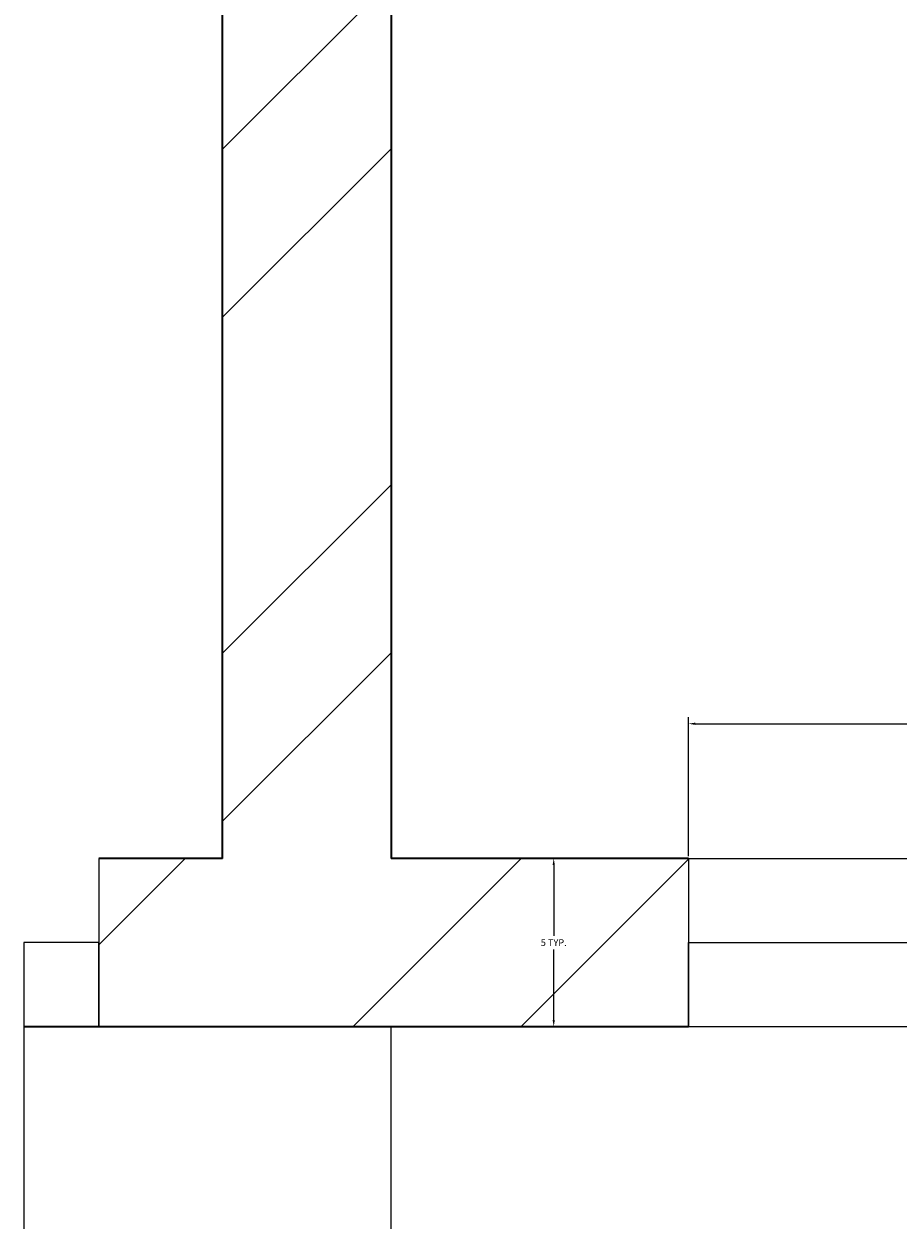
# Model space of a CAD drawing. Units: inches. Extents: x 1885 to 2748, y 783 to 2421.
# Tile 16 of 117: x 2102 to 2126, y 1082 to 1114. Entities that reach past the tile are written whole.
import ezdxf

# ---------------------------------------------------------------- set-up
doc = ezdxf.new("R2010")
doc.units = ezdxf.units.IN
for name, color, linetype, lineweight in [('A-ANNO-DIMS', 2, 'Continuous', 18), ('A-DOOR', 31, 'Continuous', 18), ('A-FLOR-BALC', 7, 'Continuous', 25), ('A-GLAZ', 181, 'Continuous', 18), ('A-WALL', 7, 'Continuous', 35)]:
    doc.layers.add(name, color=color, linetype=linetype, lineweight=lineweight)
doc.layers.add('A-WALL-PATT', color=85, linetype='Continuous', lineweight=13, true_color=0x58ba48)
doc.styles.get("Standard").update_dxf_attribs({"font": 'arial.ttf'})
doc.dimstyles.get("Standard").update_dxf_attribs({"dimtxt": 0.18, "dimasz": 0.18, "dimexe": 0.18, "dimexo": 0.0625, "dimgap": 0.09, "dimtad": 0, "dimtih": 1, "dimtoh": 1, "dimdec": 4, "dimzin": 0, "dimdsep": 46, "dimtxsty": 'Standard', "dimcen": 0.09, "dimadec": 0, "dimazin": 0, "dimtfac": 1, "dimtdec": 4, "dimtofl": 0, "dimtmove": 0, "dimatfit": 3, "dimfxl": 1, "dimtolj": 1, "dimtzin": 0, "dimarcsym": 0})

# ---------------------------------------------------------------- blocks, each defined once
blk = doc.blocks.new('WIN-24')
for p, q in [((0.001, 4.496), (0.001, -0.004)), ((0.001, 4.496), (24.001, 4.496)), ((24.001, 2.246), (24.001, 4.496)), ((24.001, 4.496), (24.001, -0.004)), ((0.001, -0.004), (0.001, 2.246)), ((0.001, 2.246), (24.001, 2.246)), ((24.001, -0.004), (0.001, -0.004))]:
    blk.add_line(p, q)
blk = doc.blocks.new('*D23')
at = {"layer": 'A-ANNO-DIMS', "color": 0, "lineweight": -2, "transparency": 16777216}
for p, q in [((2120.221, 1092.068), (2120.221, 1095.786)), ((2144.221, 1092.068), (2144.221, 1095.786)), ((2120.401, 1095.606), (2131.102, 1095.606)), ((2144.041, 1095.606), (2133.339, 1095.606))]:
    blk.add_line(p, q, dxfattribs=at)
at = {"layer": 'A-ANNO-DIMS', "color": 0, "transparency": 16777216}
for points in [[(2120.401, 1095.636), (2120.401, 1095.576), (2120.221, 1095.606)], [(2144.041, 1095.636), (2144.041, 1095.576), (2144.221, 1095.606)]]:
    blk.add_solid(points, dxfattribs=at)
at = {"layer": 'Defpoints', "color": 0, "transparency": 16777216}
for p in [(2144.221, 1095.606), (2120.221, 1092.006), (2144.221, 1092.006)]:
    blk.add_point(p, dxfattribs=at)
at = {"layer": 'A-ANNO-DIMS', "color": 0, "transparency": 16777216, "insert": (2132.221, 1095.606), "char_height": 0.18, "attachment_point": 5}
blk.add_mtext('\\A1;WINDOW 24 TYP.', dxfattribs=at)
blk = doc.blocks.new('*D24')
at = {"layer": 'A-ANNO-DIMS', "color": 0, "lineweight": -2, "transparency": 16777216}
for p, q in [((2120.158, 1092.006), (2116.441, 1092.006)), ((2116.621, 1091.826), (2116.621, 1089.937)), ((2116.621, 1087.686), (2116.621, 1089.574)), ((2120.158, 1087.506), (2116.441, 1087.506))]:
    blk.add_line(p, q, dxfattribs=at)
at = {"layer": 'A-ANNO-DIMS', "color": 0, "transparency": 16777216}
for points in [[(2116.591, 1091.826), (2116.651, 1091.826), (2116.621, 1092.006)], [(2116.591, 1087.686), (2116.651, 1087.686), (2116.621, 1087.506)]]:
    blk.add_solid(points, dxfattribs=at)
at = {"layer": 'Defpoints', "color": 0, "transparency": 16777216}
for p in [(2116.621, 1092.006), (2120.221, 1092.006), (2120.221, 1087.506)]:
    blk.add_point(p, dxfattribs=at)
at = {"layer": 'A-ANNO-DIMS', "color": 0, "transparency": 16777216, "insert": (2116.621, 1089.756), "char_height": 0.18, "attachment_point": 5}
blk.add_mtext('\\A1;5 TYP.', dxfattribs=at)

msp = doc.modelspace()

# ---------------------------------------------------------------- hatches: boundary and pattern name
at = {"layer": 'A-WALL-PATT'}
h = msp.add_hatch(dxfattribs=at)
h.set_pattern_fill('ANSI32', color=256)
h.paths.add_polyline_path([(2007.772, 2318.006), (1980.774, 2318.006), (1980.774, 2281.215), (1985.274, 2281.215), (1985.274, 2313.506), (2007.772, 2313.506), (2007.772, 2315.756)])
h.paths.add_polyline_path([(2094.324, 2318.006), (2067.772, 2318.006), (2067.772, 2313.506), (2094.324, 2313.506), (2094.324, 2315.756)])
h.paths.add_polyline_path([(2131.367, 2315.756), (2131.367, 2318.006), (2131.189, 2318.006), (2112.609, 2318.006), (2112.609, 2313.506), (2117.274, 2313.506), (2117.274, 2255.201), (2121.774, 2255.201), (2121.774, 2313.506), (2131.367, 2313.506)])
h.paths.add_polyline_path([(2190.512, 2318.006), (2155.367, 2318.006), (2155.367, 2313.506), (2169.774, 2313.506), (2169.774, 2229.506), (2121.774, 2229.506), (2121.774, 2233.451), (2119.524, 2233.451), (2117.274, 2233.451), (2117.274, 2201.101), (2121.774, 2201.101), (2121.774, 2225.006), (2169.774, 2225.006), (2169.774, 2165.006), (2306.274, 2165.006), (2306.274, 2066.006), (2310.774, 2066.006), (2344.274, 2066.006), (2486.274, 2066.006), (2486.274, 1886.006), (2483.02, 1886.006), (2483.02, 1881.506), (2486.274, 1881.506), (2486.274, 1880.678), (2490.774, 1880.678), (2490.774, 2070.506), (2344.274, 2070.506), (2310.774, 2070.506), (2310.774, 2165.006), (2310.774, 2173.636), (2308.524, 2173.636), (2306.274, 2173.636), (2306.274, 2169.506), (2174.274, 2169.506), (2174.274, 2313.506), (2190.512, 2313.506), (2190.512, 2315.756)])
h.paths.add_polyline_path([(1985.274, 2221.215), (1980.774, 2221.215), (1980.774, 2165.006), (1992.774, 2165.006), (1992.774, 2141.927), (1997.274, 2141.927), (1997.274, 2165.006), (2117.274, 2165.006), (2117.274, 2163.126), (2121.774, 2163.126), (2121.774, 2172.734), (2119.524, 2172.734), (2117.274, 2172.734), (2117.274, 2169.506), (1985.274, 2169.506)])
h.paths.add_polyline_path([(1997.274, 2105.927), (1992.774, 2105.927), (1992.774, 2070.506), (2016.774, 2070.506), (2016.774, 2059.123), (2019.024, 2059.123), (2021.274, 2059.123), (2021.274, 2070.506), (2117.274, 2070.506), (2117.274, 2022.506), (2114.423, 2022.506), (2114.423, 2018.006), (2123.627, 2018.006), (2123.627, 2020.256), (2123.627, 2022.506), (2121.774, 2022.506), (2121.774, 2142.587), (2119.524, 2142.587), (2117.274, 2142.587), (2117.274, 2075.006), (1997.274, 2075.006)])
h.paths.add_polyline_path([(2092.029, 2020.256), (2092.029, 2022.506), (2021.274, 2022.506), (2021.274, 2035.123), (2016.774, 2035.123), (2016.774, 2018.006), (2016.774, 1978.784), (2021.274, 1978.784), (2021.274, 2018.006), (2092.029, 2018.006)])
h.paths.add_polyline_path([(2260.938, 2022.506), (2153.105, 2022.506), (2153.105, 2020.256), (2153.105, 2018.006), (2155.274, 2018.006), (2155.274, 1886.006), (2107.629, 1886.006), (2107.629, 1881.506), (2182.911, 1881.506), (2182.911, 1883.756), (2182.911, 1886.006), (2159.774, 1886.006), (2159.774, 2018.006), (2260.938, 2018.006), (2260.938, 2020.256)])
h.paths.add_polyline_path([(2047.629, 1883.756), (2047.629, 1886.006), (2021.274, 1886.006), (2021.274, 1918.784), (2019.024, 1918.784), (2016.774, 1918.784), (2016.774, 1881.506), (2047.629, 1881.506)])
h.paths.add_polyline_path([(2306.361, 1883.756), (2306.361, 1886.006), (2296.274, 1886.006), (2296.274, 1982.006), (2316.535, 1982.006), (2316.535, 1984.256), (2316.535, 1986.506), (2296.274, 1986.506), (2296.274, 2022.506), (2289.276, 2022.506), (2289.276, 2018.006), (2291.774, 2018.006), (2291.774, 1886.006), (2242.911, 1886.006), (2242.911, 1881.506), (2306.361, 1881.506)], flags=17)
h.paths.add_polyline_path([(1985.274, 1843.006), (2021.6, 1843.006), (2021.534, 1845.441), (2021.477, 1847.506), (1980.774, 1847.506), (1980.774, 1809.446), (1985.274, 1809.446)])
h.paths.add_polyline_path([(2131.482, 1845.256), (2131.482, 1847.506), (2081.534, 1847.506), (2081.534, 1843.006), (2117.274, 1843.006), (2117.274, 1784.147), (2119.524, 1784.147), (2121.774, 1784.147), (2121.774, 1843.006), (2131.482, 1843.006)])
h.paths.add_polyline_path([(2203.886, 1847.506), (2155.482, 1847.506), (2155.482, 1843.006), (2169.774, 1843.006), (2169.774, 1759.006), (2121.774, 1759.006), (2121.774, 1761.457), (2117.274, 1761.457), (2117.274, 1730.429), (2121.774, 1730.429), (2121.774, 1754.506), (2177.421, 1754.506), (2177.421, 1756.756), (2177.421, 1759.006), (2174.274, 1759.006), (2174.274, 1843.006), (2203.886, 1843.006)])
h.paths.add_polyline_path([(2335.554, 1845.256), (2335.554, 1847.506), (2239.886, 1847.506), (2239.886, 1843.006), (2306.274, 1843.006), (2306.274, 1759.006), (2199.486, 1759.006), (2199.486, 1754.506), (2310.774, 1754.506), (2310.774, 1843.006), (2335.554, 1843.006)])
h.paths.add_polyline_path([(2348.774, 2022.506), (2344.274, 2022.506), (2344.274, 1986.506), (2341.681, 1986.506), (2341.681, 1982.006), (2344.274, 1982.006), (2344.274, 1886.006), (2330.361, 1886.006), (2330.361, 1881.506), (2361.627, 1881.506), (2361.627, 1883.756), (2361.627, 1886.006), (2348.774, 1886.006)], flags=17)
h.paths.add_polyline_path([(2283.251, 2315.756), (2283.251, 2318.006), (2238.512, 2318.006), (2238.512, 2313.506), (2283.251, 2313.506)], flags=17)
h.paths.add_polyline_path([(2363.274, 2348.006), (2388.677, 2348.006), (2388.677, 2350.256), (2388.677, 2352.506), (2358.774, 2352.506), (2358.774, 2348.006), (2358.774, 2318.006), (2344.481, 2318.006), (2344.481, 2313.506), (2358.774, 2313.506), (2358.774, 2229.506), (2310.774, 2229.506), (2310.774, 2231.952), (2306.274, 2231.952), (2306.274, 2205.611), (2310.774, 2205.611), (2310.774, 2225.006), (2358.774, 2225.006), (2358.774, 2211.506), (2452.329, 2211.506), (2452.329, 2213.756), (2452.329, 2216.006), (2363.274, 2216.006), (2363.274, 2318.006)])
h.paths.add_polyline_path([(2310.774, 2313.506), (2320.481, 2313.506), (2320.481, 2315.756), (2320.481, 2318.006), (2302.728, 2318.006), (2302.728, 2313.506), (2306.274, 2313.506), (2306.274, 2251.076), (2310.774, 2251.076)], flags=17)
h.paths.add_polyline_path([(2490.774, 2352.506), (2486.274, 2352.506), (2448.677, 2352.506), (2448.677, 2348.006), (2486.274, 2348.006), (2486.274, 2318.006), (2486.274, 2216.006), (2481.78, 2216.006), (2481.78, 2211.506), (2486.274, 2211.506), (2486.274, 2165.006), (2493.289, 2165.006), (2493.289, 2167.256), (2493.289, 2169.506), (2490.774, 2169.506), (2490.774, 2313.506), (2494.429, 2313.506), (2494.429, 2318.006), (2490.774, 2318.006)])
h.paths.add_polyline_path([(2534.653, 2318.006), (2515.691, 2318.006), (2515.691, 2313.506), (2534.653, 2313.506), (2534.653, 2315.756)])
h.paths.add_polyline_path([(2618.274, 2318.006), (2594.653, 2318.006), (2594.653, 2313.506), (2613.774, 2313.506), (2613.774, 2281.706), (2618.274, 2281.706)])
h.paths.add_polyline_path([(2618.274, 2221.706), (2613.774, 2221.706), (2613.774, 2169.506), (2554.019, 2169.506), (2554.019, 2165.006), (2613.774, 2165.006), (2613.774, 2152.878), (2618.274, 2152.878)])
h.paths.add_polyline_path([(2618.274, 2128.878), (2616.024, 2128.878), (2613.774, 2128.878), (2613.774, 2117.006), (2529.774, 2117.006), (2529.774, 2165.006), (2532.848, 2165.006), (2532.848, 2169.506), (2522.867, 2169.506), (2522.867, 2165.006), (2525.274, 2165.006), (2525.274, 2117.006), (2525.274, 2112.506), (2525.274, 2108.576), (2529.774, 2108.576), (2529.774, 2112.506), (2613.774, 2112.506), (2613.774, 2080.19), (2618.274, 2080.19)])
h.paths.add_polyline_path([(2618.274, 2044.19), (2616.024, 2044.19), (2613.774, 2044.19), (2613.774, 2015.506), (2529.774, 2015.506), (2529.774, 2088.582), (2527.524, 2088.582), (2525.274, 2088.582), (2525.274, 2011.006), (2613.774, 2011.006), (2613.774, 1956.755), (2618.274, 1956.755)])
h.paths.add_polyline_path([(2618.274, 1881.506), (2618.274, 1896.755), (2613.774, 1896.755), (2613.774, 1881.506), (2613.774, 1847.506), (2592.715, 1847.506), (2592.715, 1843.006), (2613.774, 1843.006), (2613.774, 1765.006), (2613.774, 1760.506), (2609.621, 1760.506), (2609.621, 1756.006), (2613.774, 1756.006), (2613.774, 1660.006), (2608.544, 1660.006), (2608.544, 1655.506), (2613.774, 1655.506), (2613.774, 1508.158), (2618.274, 1508.158)])
h.paths.add_polyline_path([(2565.774, 1843.006), (2568.997, 1843.006), (2568.997, 1847.506), (2490.774, 1847.506), (2490.774, 1849.7), (2488.524, 1849.7), (2486.274, 1849.7), (2486.274, 1847.506), (2477.274, 1847.506), (2477.274, 1838.506), (2477.274, 1821.493), (2486.274, 1821.493), (2486.274, 1838.506), (2561.274, 1838.506), (2561.274, 1765.006), (2486.274, 1765.006), (2486.274, 1786.157), (2477.274, 1786.157), (2477.274, 1765.006), (2477.274, 1756.006), (2486.274, 1756.006), (2565.774, 1756.006), (2585.621, 1756.006), (2585.621, 1758.256), (2585.621, 1760.506), (2565.774, 1760.506), (2565.774, 1765.006)])
h.paths.add_polyline_path([(2486.274, 1651.006), (2561.274, 1651.006), (2561.274, 1567.006), (2486.274, 1567.006), (2486.274, 1591.321), (2477.274, 1591.321), (2477.274, 1567.006), (2477.274, 1558.006), (2477.274, 1555.439), (2481.774, 1555.439), (2481.774, 1558.006), (2568.653, 1558.006), (2568.653, 1560.256), (2568.653, 1562.506), (2565.774, 1562.506), (2565.774, 1655.506), (2584.544, 1655.506), (2584.544, 1657.756), (2584.544, 1660.006), (2565.774, 1660.006), (2486.274, 1660.006), (2477.274, 1660.006), (2477.274, 1651.006), (2477.274, 1632.989), (2486.274, 1632.989)])
h.paths.add_polyline_path([(2449.967, 1883.756), (2449.967, 1886.006), (2421.627, 1886.006), (2421.627, 1881.506), (2449.967, 1881.506)], flags=17)
h.paths.add_polyline_path([(2447.274, 1847.506), (2395.554, 1847.506), (2395.554, 1843.006), (2442.774, 1843.006), (2442.774, 1809.27), (2447.274, 1809.27)])
h.paths.add_polyline_path([(1985.274, 1749.446), (1980.774, 1749.446), (1980.774, 1694.504), (1985.274, 1694.504), (1985.274, 1694.506), (1986.897, 1694.506), (1986.897, 1697.78), (1986.897, 1699.006), (1985.274, 1699.006)])
h.paths.add_polyline_path([(2152.774, 1699.006), (2121.774, 1699.006), (2121.774, 1703.668), (2119.524, 1703.668), (2117.274, 1703.668), (2117.274, 1699.006), (2009.219, 1699.006), (2009.219, 1694.506), (2148.274, 1694.506), (2148.274, 1692.631), (2152.774, 1692.631)])
h.paths.add_polyline_path([(2016.274, 1694.506), (2011.774, 1694.506), (2011.774, 1558.006), (2040.806, 1558.006), (2040.806, 1560.256), (2040.806, 1562.506), (2016.274, 1562.506)])
h.paths.add_polyline_path([(2152.774, 1663.017), (2150.524, 1663.017), (2148.274, 1663.017), (2148.274, 1562.506), (2100.806, 1562.506), (2100.806, 1558.006), (2165.119, 1558.006), (2165.119, 1560.256), (2165.119, 1562.506), (2152.774, 1562.506), (2152.774, 1610.506), (2224.774, 1610.506), (2224.774, 1607.99), (2229.274, 1607.99), (2229.274, 1615.006), (2152.774, 1615.006)])
h.paths.add_polyline_path([(2238.613, 1560.256), (2238.613, 1562.506), (2229.274, 1562.506), (2229.274, 1588.756), (2227.024, 1588.763), (2224.774, 1588.771), (2224.774, 1562.506), (2189.119, 1562.506), (2189.119, 1558.006), (2238.613, 1558.006)])
h.paths.add_polyline_path([(2336.024, 1560.256), (2336.024, 1562.506), (2310.774, 1562.506), (2310.774, 1656.347), (2308.524, 1656.347), (2306.274, 1656.347), (2306.274, 1562.506), (2286.613, 1562.506), (2286.613, 1558.006), (2336.024, 1558.006)])
h.paths.add_polyline_path([(2447.274, 1690.968), (2445.024, 1690.968), (2442.774, 1690.968), (2442.774, 1687.006), (2306.274, 1687.006), (2306.274, 1680.75), (2310.774, 1680.75), (2310.774, 1682.506), (2442.774, 1682.506), (2442.774, 1562.506), (2396.024, 1562.506), (2396.024, 1558.006), (2447.274, 1558.006)])
h.paths.add_polyline_path([(2447.274, 1749.27), (2445.024, 1749.27), (2442.774, 1749.27), (2442.774, 1717.232), (2447.274, 1717.232)])
h.paths.add_polyline_path([(2044.674, 1521.756), (2044.674, 1524.006), (2007.274, 1524.006), (2007.274, 1503.49), (2009.524, 1503.49), (2011.774, 1503.49), (2011.774, 1519.506), (2044.674, 1519.506)])
h.paths.add_polyline_path([(2177.969, 1521.756), (2177.969, 1524.006), (2104.674, 1524.006), (2104.674, 1519.506), (2145.774, 1519.506), (2145.774, 1387.506), (2143.37, 1387.506), (2143.37, 1383.006), (2251.585, 1383.006), (2251.585, 1385.256), (2251.585, 1387.506), (2150.274, 1387.506), (2150.274, 1519.506), (2177.969, 1519.506)])
h.paths.add_polyline_path([(2298.704, 1524.006), (2237.969, 1524.006), (2237.969, 1519.506), (2282.274, 1519.506), (2282.274, 1387.506), (2279.683, 1387.506), (2279.683, 1383.006), (2286.774, 1383.006), (2286.774, 1419.006), (2312.451, 1419.006), (2312.451, 1421.256), (2312.451, 1423.506), (2286.774, 1423.506), (2286.774, 1519.506), (2298.704, 1519.506), (2298.704, 1521.722)], flags=17)
h.paths.add_polyline_path([(2361.897, 1521.756), (2361.897, 1524.006), (2322.704, 1524.006), (2322.704, 1519.506), (2334.774, 1519.506), (2334.774, 1423.506), (2331.93, 1423.506), (2331.93, 1419.006), (2334.774, 1419.006), (2334.774, 1387.506), (2334.774, 1383.228), (2339.274, 1383.228), (2339.274, 1387.506), (2339.274, 1519.506), (2361.897, 1519.506)], flags=17)
h.paths.add_polyline_path([(2447.274, 1521.756), (2447.274, 1524.006), (2421.897, 1524.006), (2421.897, 1519.506), (2447.274, 1519.506)], flags=17)
h.paths.add_polyline_path([(2481.774, 1529.6), (2479.524, 1529.6), (2477.274, 1529.6), (2477.274, 1524.006), (2474.489, 1524.006), (2474.489, 1519.506), (2477.274, 1519.506), (2477.274, 1334.506), (2296.774, 1334.506), (2296.774, 1240.506), (2160.274, 1240.506), (2160.274, 1180.506), (2112.274, 1180.506), (2112.274, 1207.692), (2110.024, 1207.692), (2107.774, 1207.692), (2107.774, 1171.609), (2112.274, 1171.609), (2112.274, 1176.006), (2160.274, 1176.006), (2160.274, 1092.006), (2144.221, 1092.006), (2144.221, 1087.506), (2189.497, 1087.506), (2189.497, 1089.756), (2189.497, 1092.006), (2164.774, 1092.006), (2164.774, 1236.006), (2296.774, 1236.006), (2296.774, 1231.912), (2301.274, 1231.912), (2301.274, 1330.006), (2481.774, 1330.006), (2481.774, 1387.506)])
h.paths.add_polyline_path([(2618.274, 1448.158), (2613.774, 1448.158), (2613.774, 1382.506), (2529.774, 1382.506), (2525.274, 1382.506), (2525.274, 1307.062), (2529.774, 1307.062), (2529.774, 1378.006), (2613.774, 1378.006), (2613.774, 1354.988), (2618.274, 1354.988)])
h.paths.add_polyline_path([(2618.274, 1318.988), (2613.774, 1318.988), (2613.774, 1281.006), (2529.774, 1281.006), (2529.774, 1283.786), (2527.524, 1283.786), (2525.274, 1283.786), (2525.274, 1228.506), (2516.794, 1228.506), (2516.794, 1224.006), (2533.484, 1224.006), (2533.484, 1226.256), (2533.484, 1228.506), (2529.774, 1228.506), (2529.774, 1276.506), (2613.774, 1276.506), (2613.774, 1266.02), (2618.274, 1266.02)])
h.paths.add_polyline_path([(2618.274, 1134.964), (2613.774, 1134.964), (2613.774, 1092.006), (2594.545, 1092.006), (2594.545, 1087.506), (2618.274, 1087.506)])
h.paths.add_polyline_path([(2534.545, 1092.006), (2509.765, 1092.006), (2509.765, 1087.506), (2534.545, 1087.506), (2534.545, 1089.756)])
h.paths.add_polyline_path([(2481.274, 1224.006), (2484.117, 1224.006), (2484.117, 1226.256), (2484.117, 1228.506), (2476.774, 1228.506), (2476.774, 1198.506), (2471.61, 1198.506), (2471.61, 1194.006), (2476.774, 1194.006), (2476.774, 1062.006), (2436.894, 1062.006), (2436.894, 1057.506), (2476.774, 1057.506), (2481.274, 1057.506), (2481.274, 1062.006), (2481.274, 1087.506), (2485.354, 1087.506), (2485.354, 1089.756), (2485.354, 1092.006), (2481.274, 1092.006), (2481.274, 1117.506)])
h.paths.add_polyline_path([(2439.898, 1198.506), (2349.274, 1198.506), (2349.274, 1194.006), (2349.274, 1180.506), (2301.274, 1180.506), (2301.274, 1201.896), (2299.024, 1201.896), (2296.774, 1201.896), (2296.774, 1172.335), (2299.024, 1172.335), (2301.274, 1172.335), (2301.274, 1176.006), (2349.274, 1176.006), (2349.274, 1092.006), (2334.452, 1092.006), (2334.452, 1087.506), (2349.274, 1087.506), (2349.274, 1057.506), (2353.774, 1057.506), (2376.894, 1057.506), (2376.894, 1059.756), (2376.894, 1062.006), (2353.774, 1062.006), (2353.774, 1087.506), (2353.774, 1180.506), (2353.774, 1194.006), (2439.898, 1194.006), (2439.898, 1196.256)])
h.paths.add_polyline_path([(2270.596, 1089.756), (2270.596, 1092.006), (2249.497, 1092.006), (2249.497, 1087.506), (2270.596, 1087.506)], flags=17)
h.paths.add_polyline_path([(2310.452, 1092.006), (2301.274, 1092.006), (2301.274, 1153.292), (2296.774, 1153.292), (2296.774, 1092.006), (2293.786, 1092.006), (2293.786, 1087.506), (2310.452, 1087.506), (2310.452, 1089.756)], flags=17)
h.paths.add_polyline_path([(2112.274, 1150.328), (2110.024, 1150.328), (2107.774, 1150.328), (2107.774, 1092.006), (2104.465, 1092.006), (2104.465, 1087.506), (2120.221, 1087.506), (2120.221, 1089.756), (2120.221, 1092.006), (2112.274, 1092.006)])
h.paths.add_polyline_path([(2082.172, 1092.006), (2058.144, 1092.006), (2058.144, 1087.506), (2082.172, 1087.506), (2082.172, 1089.756)])
h.paths.add_polyline_path([(1975.774, 1145.638), (1971.274, 1145.638), (1971.274, 1087.506), (1980.774, 1087.506), (1998.144, 1087.506), (1998.144, 1089.756), (1998.144, 1092.006), (1985.274, 1092.006), (1975.774, 1092.006)])
h.paths.add_polyline_path([(2112.274, 1244.385), (2110.024, 1244.385), (2107.774, 1244.385), (2107.774, 1240.506), (1992.274, 1240.506), (1992.274, 1271.008), (1987.774, 1271.008), (1987.774, 1240.506), (1980.774, 1240.506), (1975.774, 1240.506), (1971.274, 1240.506), (1971.274, 1205.638), (1975.774, 1205.638), (1975.774, 1236.006), (2107.774, 1236.006), (2107.774, 1233.444), (2112.274, 1233.444), (2112.274, 1236.006)])
h.paths.add_polyline_path([(2112.274, 1383.006), (2114.783, 1383.006), (2114.783, 1385.256), (2114.783, 1387.506), (2102.476, 1387.506), (2102.476, 1383.006), (2107.774, 1383.006), (2107.774, 1335.006), (2011.774, 1335.006), (2011.774, 1349.939), (2007.274, 1349.939), (2007.274, 1335.006), (1987.774, 1335.006), (1987.774, 1330.506), (1987.774, 1307.008), (1992.274, 1307.008), (1992.274, 1330.506), (2007.274, 1330.506), (2107.774, 1330.506), (2107.774, 1264.711), (2112.274, 1264.711)])
h.paths.add_polyline_path([(2077.857, 1387.506), (2011.774, 1387.506), (2011.774, 1390.036), (2009.524, 1390.036), (2007.274, 1390.036), (2007.274, 1373.939), (2011.774, 1373.939), (2011.774, 1383.006), (2077.857, 1383.006)])
h.paths.add_polyline_path([(2011.774, 1443.49), (2007.274, 1443.49), (2007.274, 1410.248), (2011.774, 1410.248)])

# ---------------------------------------------------------------- linework, layer by layer
at = {"layer": 'A-DOOR'}
for p, q in [((2104.465, 1092.006), (2104.465, 1087.506)), ((2104.465, 1089.756), (2102.465, 1089.756)), ((2102.465, 1089.756), (2102.465, 1065.756)), ((2104.465, 1087.506), (2104.465, 1089.756))]:
    msp.add_line(p, q, dxfattribs=at)
at = {"layer": 'A-FLOR-BALC'}
msp.add_line((2112.274, 1057.506), (2112.274, 1087.506), dxfattribs=at)
at = {"layer": 'A-WALL'}
for p, q in [((2112.274, 1151.733), (2112.274, 1092.006)), ((2107.774, 1092.006), (2107.774, 1150.328)), ((2107.774, 1092.006), (2104.465, 1092.006)), ((2120.221, 1092.006), (2112.274, 1092.006)), ((2120.221, 1087.506), (2102.465, 1087.506))]:
    msp.add_line(p, q, dxfattribs=at)

# ---------------------------------------------------------------- block references
at = {"layer": 'A-GLAZ'}
msp.add_blockref('WIN-24', (2120.22, 1087.51), dxfattribs=at)

# ---------------------------------------------------------------- dimensions: what is measured, and where the dimension line sits
at = {"layer": 'A-ANNO-DIMS'}
dim = msp.add_linear_dim(base=(2144.221, 1095.606), p1=(2120.221, 1092.006), p2=(2144.221, 1092.006), text='WINDOW <> TYP.', dimstyle='Standard', override={"dimdec": 0, "dimlfac": 1, "dimrnd": 0, "dimzin": 0, "dimdsep": 46, "dimlunit": 2}, dxfattribs=at)
dim.commit()
dim.dimension.update_dxf_attribs({"geometry": '*D23', "text_midpoint": (2132.221, 1095.606)})
dim = msp.add_linear_dim(base=(2116.620549077, 1092.005556822), p1=(2120.220549077, 1087.505556822), p2=(2120.220549077, 1092.005556822), angle=90, text='<> TYP.', dimstyle='Standard', override={"dimdec": 0, "dimlfac": 1, "dimrnd": 0, "dimzin": 0, "dimdsep": 46, "dimlunit": 2}, dxfattribs=at)
dim.commit()
dim.dimension.update_dxf_attribs({"geometry": '*D24', "text_midpoint": (2116.620549077, 1089.755556822)})

doc.saveas('drawing.dxf')
